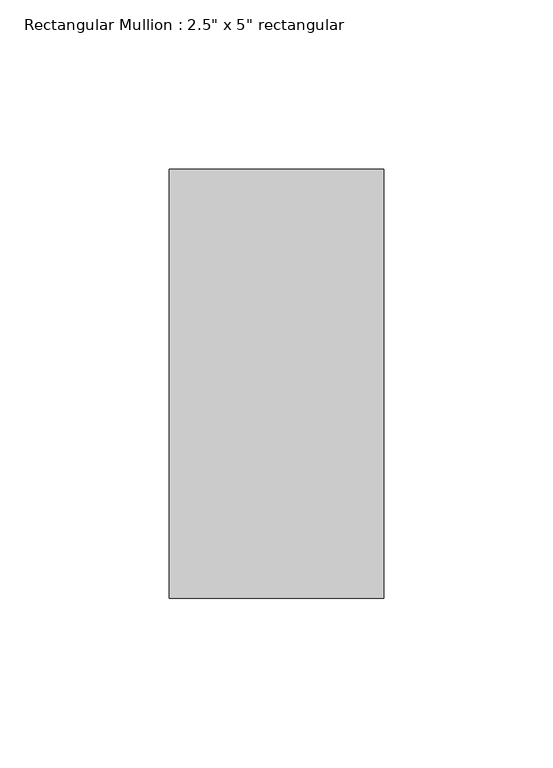
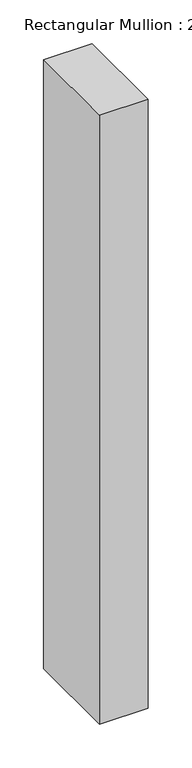
"""IFC4 building model written with IfcOpenShell, lengths in millimetres: member geometry."""

from ifc_helpers import new_model, si_unit, frame, origin, place, context, project, spatial, polyline, outline, extrude, source, transform, mapped, element, save


def member_091e92f8(model_context):
    return source(origin(), model_context, "Body", "SweptSolid", [
        extrude(outline(polyline([(0.0, 63.5), (0.0, -63.5), (-63.5, -63.5), (-63.5, 63.5), (0.0, 63.5)])), frame((0.0, 0.0, -844.55), z_axis=(0.0, 0.0, 1.0), x_axis=(1.0, 0.0, 0.0)), (0.0, 0.0, 1.0), 844.55),
    ])


if __name__ == "__main__":
    model = new_model("IFC4")
    model_context = context("Model", 3, world=origin())
    ifc_project = project(units=[si_unit("LENGTHUNIT", "METRE", prefix="MILLI")], contexts=[model_context])
    site = spatial("IfcSite", under=ifc_project)
    building = spatial("IfcBuilding", under=site)
    placement = place(None, origin())
    member_shape = member_091e92f8(model_context)
    element("IfcMember", 1, ObjectType="Rectangular Mullion : 2.5\" x 5\" rectangular", at=placement, inside=building, context=model_context, shape_type="MappedRepresentation", body=[
        mapped(member_shape, transform((0.0, 0.0, 0.0), x_axis=(1.0, 0.0, 0.0), y_axis=(0.0, 1.0, 0.0), z_axis=(0.0, 0.0, 1.0))),
    ])
    save(model, "model.ifc")

# Revit data of these elements
# Type "Rectangular Mullion : 2.5\" x 5\" rectangular"
#   built-in parameter 1007304 = 0.416667 (stored number, unit not read)
#   built-in parameter 1007301 = 0.104167 (stored number, unit not read)
#   built-in parameter 1007300 = 0.104167 (stored number, unit not read)
# Element 1 (IfcMember, "Rectangular Mullion : 2.5\" x 5\" rectangular")
#   Materials on its faces: "Aluminum"
# Materials
#   "Aluminum": class "Metal", colour RGB 247 247 247, transparency 0, Description = "Aluminum 6061", Cost = 0
